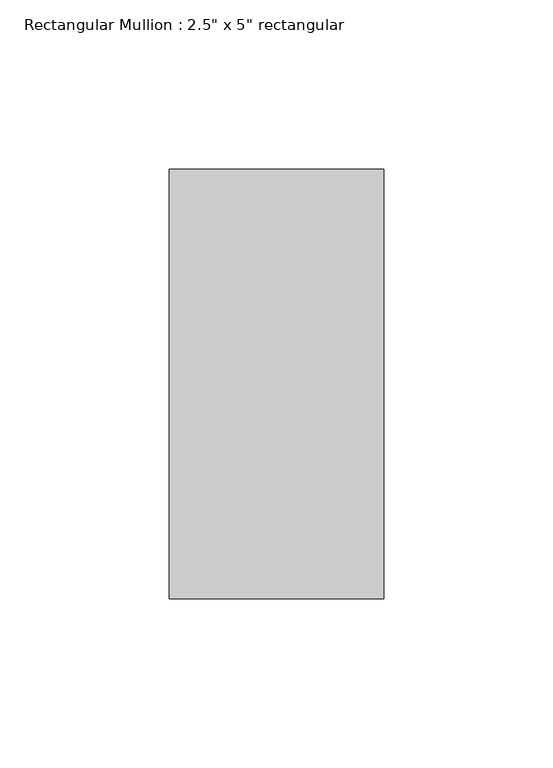
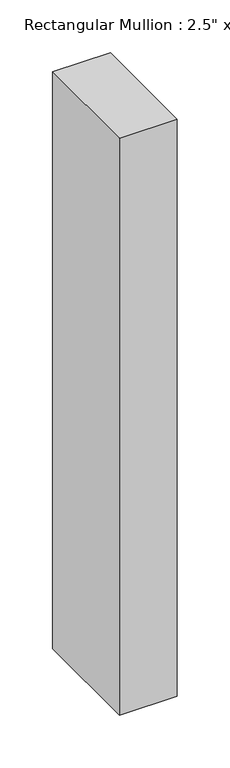
"""IFC4 building model written with IfcOpenShell, lengths in millimetres: member geometry."""

from ifc_helpers import new_model, si_unit, frame, origin, place, context, project, spatial, polyline, outline, extrude, source, transform, mapped, element, save


def member_377cf5f8(model_context):
    return source(origin(), model_context, "Body", "SweptSolid", [
        extrude(outline(polyline([(0.0, 63.5), (0.0, -63.5), (-63.5, -63.5), (-63.5, 63.5), (0.0, 63.5)])), frame((0.0, 0.0, -668.7147936), z_axis=(0.0, 0.0, 1.0), x_axis=(1.0, 0.0, 0.0)), (0.0, 0.0, 1.0), 668.7147936),
    ])


if __name__ == "__main__":
    model = new_model("IFC4")
    model_context = context("Model", 3, world=origin())
    ifc_project = project(units=[si_unit("LENGTHUNIT", "METRE", prefix="MILLI")], contexts=[model_context])
    site = spatial("IfcSite", under=ifc_project)
    building = spatial("IfcBuilding", under=site)
    placement = place(None, origin())
    member_shape = member_377cf5f8(model_context)
    element("IfcMember", 1, ObjectType="Rectangular Mullion : 2.5\" x 5\" rectangular", at=placement, inside=building, context=model_context, shape_type="MappedRepresentation", body=[
        mapped(member_shape, transform((0.0, 0.0, 0.0), x_axis=(1.0, 0.0, 0.0), y_axis=(0.0, 1.0, 0.0), z_axis=(0.0, 0.0, 1.0))),
    ])
    save(model, "model.ifc")

# Revit data of these elements
# Type "Rectangular Mullion : 2.5\" x 5\" rectangular"
#   built-in parameter 1007304 = 0.416667 (stored number, unit not read)
#   built-in parameter 1007301 = 0.104167 (stored number, unit not read)
#   built-in parameter 1007300 = 0.104167 (stored number, unit not read)
# Element 1 (IfcMember, "Rectangular Mullion : 2.5\" x 5\" rectangular")
#   Materials on its faces: "Aluminum"
# Materials
#   "Aluminum": class "Metal", colour RGB 247 247 247, transparency 0, Description = "Aluminum 6061", Cost = 0
